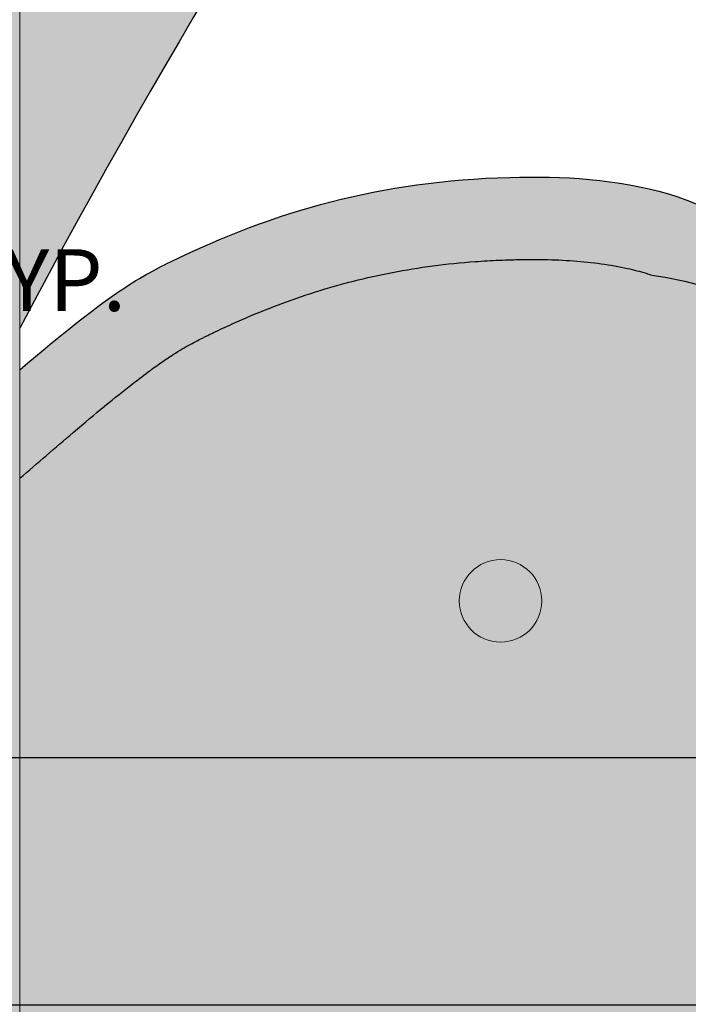
# Model space of a CAD drawing. Units: millimetres. Extents: x 11032 to 26788, y 3406 to 24505.
# Tile 72 of 78: x 22897 to 24519, y 12721 to 15110. Entities that reach past the tile are written whole.
import ezdxf

# ---------------------------------------------------------------- set-up
doc = ezdxf.new("R2010")
doc.units = ezdxf.units.MM
doc.header["$MEASUREMENT"] = 0
for name, color, linetype, lineweight in [('A-ANNO-DIMS', 2, 'Continuous', 18), ('A-GLAZ', 250, 'Continuous', 20), ('A-ROOF', 7, 'Continuous', 30), ('E-LITE', 7, 'Continuous', 18), ('E-LITE-PATT', 7, 'Continuous', 13)]:
    doc.layers.add(name, color=color, linetype=linetype, lineweight=lineweight)
for name, color, linetype, lineweight, true_color in [('A-GLAZ-FRAM-PATT', 250, 'Continuous', 13, 0x262627), ('A-ROOF-PATT', 9, 'Continuous', 13, 0xc7c8ca), ('A-WALL-CLAD-PATT', 9, 'Continuous', 13, 0xc7c8ca)]:
    doc.layers.add(name, color=color, linetype=linetype, lineweight=lineweight, true_color=true_color)
doc.styles.get("Standard").update_dxf_attribs({"font": 'arial.ttf'})
doc.dimstyles.get("Standard").update_dxf_attribs({"dimtxt": 150, "dimasz": 100, "dimexe": 10, "dimexo": 5, "dimgap": 5, "dimtad": 0, "dimtih": 1, "dimtoh": 1, "dimdec": 0, "dimzin": 0, "dimdsep": 46, "dimtxsty": 'Standard', "dimcen": 0.09, "dimadec": 0, "dimazin": 0, "dimtfac": 1, "dimtdec": 0, "dimtofl": 0, "dimtmove": 0, "dimatfit": 3, "dimfxl": 1, "dimtolj": 1, "dimtzin": 0, "dimarcsym": 0})

# ---------------------------------------------------------------- blocks, each defined once
blk = doc.blocks.new('RECESSED-LIGHT-200')
blk.add_circle((100, 100), 100)
blk = doc.blocks.new('*D20')
at = {"layer": 'A-ANNO-DIMS', "color": 0, "lineweight": -2, "transparency": 16777216}
for p, q in [((21468.9, 12413.4), (21368.9, 12413.4)), ((21568.9, 12403.4), (21568.9, 12423.4)), ((21668.9, 12403.4), (21668.9, 12423.4)), ((21768.9, 12413.4), (21868.9, 12413.4))]:
    blk.add_line(p, q, dxfattribs=at)
at = {"layer": 'A-ANNO-DIMS', "color": 0, "transparency": 16777216}
for points in [[(21468.9, 12430), (21468.9, 12396.7), (21568.9, 12413.4)], [(21768.9, 12430), (21768.9, 12396.7), (21668.9, 12413.4)]]:
    blk.add_solid(points, dxfattribs=at)
at = {"layer": 'Defpoints', "color": 0, "transparency": 16777216}
for p in [(21668.9, 12413.4), (21568.9, 12398.4), (21668.9, 12398.4)]:
    blk.add_point(p, dxfattribs=at)
at = {"layer": 'A-ANNO-DIMS', "color": 0, "transparency": 16777216, "insert": (23236.5, 12413.4), "char_height": 150, "attachment_point": 5}
blk.add_mtext('\\A1;RECESSED LIGHT 100 TYP.', dxfattribs=at)
blk = doc.blocks.new('*D22')
at = {"layer": 'A-ANNO-DIMS', "color": 0, "lineweight": -2, "transparency": 16777216}
for p, q in [((20094.7, 14478.3), (19994.7, 14478.3)), ((20194.7, 14460.8), (20194.7, 14488.3)), ((20344.7, 14460.8), (20344.7, 14488.3)), ((20444.7, 14478.3), (20544.7, 14478.3))]:
    blk.add_line(p, q, dxfattribs=at)
at = {"layer": 'A-ANNO-DIMS', "color": 0, "transparency": 16777216}
for points in [[(20094.7, 14495), (20094.7, 14461.7), (20194.7, 14478.3)], [(20444.7, 14495), (20444.7, 14461.7), (20344.7, 14478.3)]]:
    blk.add_solid(points, dxfattribs=at)
at = {"layer": 'Defpoints', "color": 0, "transparency": 16777216}
for p in [(20344.7, 14478.3), (20194.7, 14455.8), (20344.7, 14455.8)]:
    blk.add_point(p, dxfattribs=at)
at = {"layer": 'A-ANNO-DIMS', "color": 0, "transparency": 16777216, "insert": (21912.3, 14478.3), "char_height": 150, "attachment_point": 5}
blk.add_mtext('\\A1;RECESSED LIGHT 150 TYP.', dxfattribs=at)
blk = doc.blocks.new('*D36')
at = {"layer": 'A-ANNO-DIMS', "color": 0, "lineweight": -2, "transparency": 16777216}
for p, q in [((12301.3, 17115.9), (12301.3, 24416.9)), ((12401.3, 24406.9), (18569.2, 24406.9)), ((25297.4, 24406.9), (19129.5, 24406.9)), ((25397.4, 4466.4), (25397.4, 24416.9))]:
    blk.add_line(p, q, dxfattribs=at)
at = {"layer": 'A-ANNO-DIMS', "color": 0, "transparency": 16777216}
for points in [[(12401.3, 24423.5), (12401.3, 24390.2), (12301.3, 24406.9)], [(25297.4, 24423.5), (25297.4, 24390.2), (25397.4, 24406.9)]]:
    blk.add_solid(points, dxfattribs=at)
at = {"layer": 'Defpoints', "color": 0, "transparency": 16777216}
for p in [(25397.4, 24406.9), (12301.3, 17110.9), (25397.4, 4461.4)]:
    blk.add_point(p, dxfattribs=at)
at = {"layer": 'A-ANNO-DIMS', "color": 0, "transparency": 16777216, "insert": (18849.3, 24406.9), "char_height": 150, "attachment_point": 5}
blk.add_mtext('\\A1;13096', dxfattribs=at)
blk = doc.blocks.new('*D42')
at = {"layer": 'A-ANNO-DIMS', "color": 0, "lineweight": -2, "transparency": 16777216}
for p, q in [((22752.4, 13320.1), (26363.9, 13320.1)), ((26353.9, 13220.1), (26353.9, 13101.7)), ((26353.9, 12820.1), (26353.9, 12938.5)), ((22752.4, 12720.1), (26363.9, 12720.1))]:
    blk.add_line(p, q, dxfattribs=at)
at = {"layer": 'A-ANNO-DIMS', "color": 0, "transparency": 16777216}
for points in [[(26337.2, 13220.1), (26370.6, 13220.1), (26353.9, 13320.1)], [(26337.2, 12820.1), (26370.6, 12820.1), (26353.9, 12720.1)]]:
    blk.add_solid(points, dxfattribs=at)
at = {"layer": 'Defpoints', "color": 0, "transparency": 16777216}
for p in [(22747.4, 13320.1), (26353.9, 13320.1), (22747.4, 12720.1)]:
    blk.add_point(p, dxfattribs=at)
at = {"layer": 'A-ANNO-DIMS', "color": 0, "transparency": 16777216, "insert": (26353.9, 13020.1), "char_height": 150, "attachment_point": 5}
blk.add_mtext('\\A1;600', dxfattribs=at)
blk = doc.blocks.new('*D43')
at = {"layer": 'A-ANNO-DIMS', "color": 0, "lineweight": -2, "transparency": 16777216}
for p, q in [((22752.4, 15170.1), (26363.9, 15170.1)), ((26353.9, 15070.1), (26353.9, 14326.7)), ((26353.9, 13420.1), (26353.9, 14163.5)), ((22752.4, 13320.1), (26363.9, 13320.1))]:
    blk.add_line(p, q, dxfattribs=at)
at = {"layer": 'A-ANNO-DIMS', "color": 0, "transparency": 16777216}
for points in [[(26337.2, 15070.1), (26370.6, 15070.1), (26353.9, 15170.1)], [(26337.2, 13420.1), (26370.6, 13420.1), (26353.9, 13320.1)]]:
    blk.add_solid(points, dxfattribs=at)
at = {"layer": 'Defpoints', "color": 0, "transparency": 16777216}
for p in [(22747.4, 15170.1), (26353.9, 15170.1), (22747.4, 13320.1)]:
    blk.add_point(p, dxfattribs=at)
at = {"layer": 'A-ANNO-DIMS', "color": 0, "transparency": 16777216, "insert": (26353.9, 14245.1), "char_height": 150, "attachment_point": 5}
blk.add_mtext('\\A1;1850', dxfattribs=at)

msp = doc.modelspace()

# ---------------------------------------------------------------- hatches: boundary and pattern name
at = {"layer": 'A-GLAZ-FRAM-PATT'}
h = msp.add_hatch(color=256, dxfattribs=at)
h.paths.add_polyline_path([(22747.404, 16218.44), (22395.025, 16218.44), (18518.2, 16200.148), (18519.143, 16000.151), (22747.404, 16020.1)])
edge = h.paths.add_edge_path()
edge.add_line((22897.404, 16218.44), (22747.404, 16218.44))
edge.add_line((22747.404, 16218.44), (22747.404, 16020.1))
edge.add_line((22747.404, 16020.1), (22747.404, 9631.346))
edge.add_spline(control_points=[(22747.404, 9631.346), (22803.273, 9520.228), (22853.467, 9405.87), (22897.404, 9289.211)], knot_values=[2645.78092422, 2645.78092422, 2645.78092422, 2645.78092422, 3013.05623672, 3013.05623672, 3013.05623672, 3013.05623672], degree=3, periodic=0)
edge.add_line((22897.404, 9289.211), (22897.404, 16218.44))
h.paths.add_polyline_path([(22097.404, 16017.033), (21997.404, 16016.562), (21997.404, 13316.532), (22097.404, 13317.003)])
edge = h.paths.add_edge_path()
edge.add_line((19797.404, 16006.182), (19697.404, 16005.71))
edge.add_line((19697.404, 16005.71), (19697.404, 15155.703))
edge.add_line((19697.404, 15155.703), (19697.404, 12747.012))
edge.add_spline(control_points=[(19697.404, 12747.012), (19708.389, 12750.081), (19719.253, 12753.406), (19732.457, 12757.789), (19734.918, 12758.62), (19737.372, 12759.464)], knot_values=[1372.60477099, 1372.60477099, 1372.60477099, 1372.60477099, 1399.44343377, 1399.44343377, 1405.61279972, 1405.61279972, 1405.61279972, 1405.61279972], degree=3, periodic=0)
edge.add_spline(control_points=[(19737.372, 12759.464), (19750.245, 12763.891), (19762.932, 12768.657), (19778.9, 12775.14), (19782.354, 12776.572), (19785.794, 12778.028)], knot_values=[1405.61279972, 1405.61279972, 1405.61279972, 1405.61279972, 1437.96891336, 1437.96891336, 1446.94640473, 1446.94640473, 1446.94640473, 1446.94640473], degree=3, periodic=0)
edge.add_spline(control_points=[(19785.794, 12778.028), (19789.682, 12779.673), (19793.552, 12781.348), (19797.404, 12783.051)], knot_values=[1446.94640473, 1446.94640473, 1446.94640473, 1446.94640473, 1457.09545574, 1457.09545574, 1457.09545574, 1457.09545574], degree=3, periodic=0)
edge.add_line((19797.404, 12783.051), (19797.404, 15306.174))
edge.add_line((19797.404, 15306.174), (19797.404, 16006.182))
at = {"layer": 'A-ROOF-PATT'}
h = msp.add_hatch(color=256, dxfattribs=at)
h.set_gradient(color1=(254, 234, 185), color2=(254, 204, 102), name='HEMISPHERICAL')
edge = h.paths.add_edge_path()
edge.add_line((22395.025, 16218.44), (22897.404, 16218.44))
edge.add_line((22897.404, 16218.44), (22897.404, 14361.22))
edge.add_spline(control_points=[(22897.404, 14361.22), (23633.498, 15762.375), (24369.592, 16638.387), (24279.347, 17098.191)], knot_values=[13837.11981978, 13837.11981978, 13837.11981978, 13837.11981978, 16370.50452639, 16370.50452639, 16370.50452639, 16370.50452639], degree=3, periodic=0)
edge.add_spline(control_points=[(24279.347, 17098.191), (24257.37, 17136.735), (24193.084, 17226.949), (23988.629, 17323.661), (23687.5, 17400.339), (23443.416, 17391.278), (23304.873, 17403.391)], knot_values=[0, 0, 0, 0, 132.15616417, 336.8260172, 651.2646938, 1064.01641738, 1064.01641738, 1064.01641738, 1064.01641738], degree=3, periodic=0)
edge.add_spline(control_points=[(23304.873, 17403.391), (23244.326, 17403.734), (23179.968, 17412.17), (23070.675, 17406.134), (23026.355, 17412.719), (22981.194, 17409.426)], knot_values=[11756.28081343, 11756.28081343, 11756.28081343, 11756.28081343, 11943.0031739, 11943.0031739, 12065.87545546, 12065.87545546, 12065.87545546, 12065.87545546], degree=3, periodic=0)
edge.add_spline(control_points=[(22981.194, 17409.426), (22912.577, 17410.967), (22705.353, 17409.356), (22364.272, 17406.622), (21915.866, 17351.508), (21440.234, 17310.172), (20910.567, 17150.246), (20408.011, 17091.181), (20122.484, 17046.068), (19965.955, 17031.58)], knot_values=[0, 0, 0, 0, 192.80748108, 571.75839709, 1088.96543094, 1535.73720072, 2007.04970373, 2677.45974628, 3092.27759325, 3092.27759325, 3092.27759325, 3092.27759325], degree=3, periodic=0)
edge.add_spline(control_points=[(19965.955, 17031.58), (19761.843, 17020.464), (19288.07, 16988.339), (18809.773, 17038.521), (18514.126, 17063.566)], knot_values=[0, 0, 0, 0, 511.7030916, 1383.18424693, 1383.18424693, 1383.18424693, 1383.18424693], degree=3, periodic=0)
edge.add_line((18514.126, 17063.566), (18518.2, 16200.148))
edge.add_line((18518.2, 16200.148), (22395.025, 16218.44))
h.paths.add_polyline_path([(20159.481, 16629.671, -1), (20359.481, 16629.671, -1)], flags=16)
h.paths.add_polyline_path([(22641.869, 16640.848, -1), (22441.869, 16640.848, -1)], flags=16)
h.paths.add_polyline_path([(23436.23, 16026.079, -1), (23236.23, 16026.079, -1)], flags=16)
h = msp.add_hatch(color=256, dxfattribs=at)
h.set_gradient(color1=(254, 234, 185), color2=(254, 204, 102), name='HEMISPHERICAL')
edge = h.paths.add_edge_path()
edge.add_spline(control_points=[(22897.404, 11669.966), (22905.925, 11665.421), (23315.936, 11448.075), (24040.798, 11159.928), (24591.756, 12047.169), (24823.737, 12810.982), (24947.403, 13888.961), (24865.187, 14241.353)], knot_values=[3287.74811127, 3287.74811127, 3287.74811127, 3287.74811127, 3313.95061448, 4543.69878516, 5160.49832431, 6201.61230094, 7164.26935092, 7164.26935092, 7164.26935092, 7164.26935092], degree=3, periodic=0)
edge.add_spline(control_points=[(24865.187, 14241.353), (24864.423, 14242.575), (24766.311, 14398.016), (24602.876, 14465.087), (24430.499, 14490.269)], knot_values=[2462.20964139, 2462.20964139, 2462.20964139, 2462.20964139, 2466.8266732, 3052.28296943, 3052.28296943, 3052.28296943, 3052.28296943], degree=3, periodic=0)
edge.add_spline(control_points=[(24430.499, 14490.269), (24425.883, 14491.82), (24421.191, 14493.323), (24402.038, 14499.174), (24386.985, 14503.129), (24351.089, 14511.181), (24329.855, 14514.969), (24285.944, 14521.074), (24263.27, 14523.392), (24216.998, 14526.696), (24193.401, 14527.682), (24156.534, 14528.34), (24143.408, 14528.404), (24117.112, 14528.234), (24103.938, 14528.001), (24070.613, 14527.088), (24050.758, 14526.245), (24021.415, 14524.553), (24011.706, 14523.918), (23966.994, 14520.648), (23932.846, 14517.154), (23866.075, 14508.38), (23833.453, 14503.099), (23769.399, 14490.798), (23737.967, 14483.778), (23675.954, 14468.02), (23645.373, 14459.282), (23584.735, 14440.092), (23554.677, 14429.638), (23494.779, 14407.002), (23464.938, 14394.819), (23420.13, 14375.236), (23405.186, 14368.49), (23382.735, 14358.043), (23375.245, 14354.506), (23363.999, 14349.118), (23360.248, 14347.308), (23354.645, 14344.586), (23352.794, 14343.684), (23350.017, 14342.326), (23349.099, 14341.876), (23346.705, 14340.7), (23345.24, 14339.978), (23338.743, 14336.765), (23333.903, 14334.336), (23322.952, 14328.714), (23316.906, 14325.517), (23304.544, 14318.72), (23298.224, 14315.118), (23284.755, 14307.106), (23277.606, 14302.694), (23262.032, 14292.682), (23253.61, 14287.081), (23235.154, 14274.351), (23225.122, 14267.224), (23200.911, 14249.486), (23186.304, 14238.46), (23150.266, 14210.435), (23128.041, 14192.649), (23080.227, 14153.32), (23055.083, 14132.223), (23027.357, 14108.523)], knot_values=[765.02120011, 765.02120011, 765.02120011, 765.02120011, 788.26421035, 788.26421035, 858.47024111, 858.47024111, 949.55129088, 949.55129088, 1040.63234064, 1040.63234064, 1131.71339041, 1131.71339041, 1181.69353236, 1181.69353236, 1231.67367431, 1231.67367431, 1308.31901537, 1308.31901537, 1346.64168591, 1346.64168591, 1486.09404767, 1486.09404767, 1625.54640943, 1625.54640943, 1764.99877119, 1764.99877119, 1904.45113295, 1904.45113295, 2043.90349471, 2043.90349471, 2183.35585648, 2183.35585648, 2253.08203736, 2253.08203736, 2287.9451278, 2287.9451278, 2305.37667302, 2305.37667302, 2313.97014819, 2313.97014819, 2318.26688578, 2318.26688578, 2325.26983634, 2325.26983634, 2349.68341829, 2349.68341829, 2381.60377634, 2381.60377634, 2413.52413439, 2413.52413439, 2445.44449243, 2445.44449243, 2477.36485048, 2477.36485048, 2509.28520853, 2509.28520853, 2547.80727814, 2547.80727814, 2595.07704725, 2595.07704725, 2638.35089074, 2638.35089074, 2638.35089074, 2638.35089074], degree=3, periodic=0)
edge.add_spline(control_points=[(23027.357, 14108.523), (23027.349, 14108.516), (23027.342, 14108.51), (23027.334, 14108.504), (22984.024, 14071.482), (22940.714, 14034.46), (22897.404, 13997.439)], knot_values=[697.41436256, 697.41436256, 697.41436256, 697.41436256, 697.4261083, 697.4261083, 697.4261083, 765.02120011, 765.02120011, 765.02120011, 765.02120011], degree=3, periodic=0)
edge.add_line((22897.404, 13997.439), (22897.404, 11669.966))
h.paths.add_polyline_path([(23729.349, 12537.488, -1), (23529.349, 12537.488, -1)], flags=16)
h.paths.add_polyline_path([(23963.611, 13699.89, -1), (24163.611, 13699.89, -1)], flags=16)
at = {"layer": 'A-WALL-CLAD-PATT'}
h = msp.add_hatch(color=256, dxfattribs=at)
edge = h.paths.add_edge_path()
edge.add_spline(control_points=[(24865.187, 14241.353), (24844.683, 14329.238), (24708.481, 14689.762), (23980.011, 14777.842), (23439.65, 14624.598), (23111.535, 14443.589), (22897.404, 14260.55)], knot_values=[765.02120011, 765.02120011, 765.02120011, 765.02120011, 1005.10337375, 1880.54593672, 2963.32805357, 3287.74811127, 3287.74811127, 3287.74811127, 3287.74811127], degree=3, periodic=0)
edge.add_line((22897.404, 14260.55), (22897.404, 13997.439))
edge.add_spline(control_points=[(22897.404, 13997.439), (22940.714, 14034.46), (22984.024, 14071.482), (23027.334, 14108.504), (23027.342, 14108.51), (23027.349, 14108.516), (23027.357, 14108.523)], knot_values=[697.41436256, 697.41436256, 697.41436256, 697.41436256, 765.00945437, 765.00945437, 765.00945437, 765.02120011, 765.02120011, 765.02120011, 765.02120011], degree=3, periodic=0)
edge.add_spline(control_points=[(23027.357, 14108.523), (23055.083, 14132.223), (23080.227, 14153.32), (23128.041, 14192.649), (23150.266, 14210.435), (23186.304, 14238.46), (23200.911, 14249.486), (23225.122, 14267.224), (23235.154, 14274.351), (23253.61, 14287.081), (23262.032, 14292.682), (23277.606, 14302.694), (23284.755, 14307.106), (23298.224, 14315.118), (23304.544, 14318.72), (23316.906, 14325.517), (23322.952, 14328.714), (23333.903, 14334.336), (23338.743, 14336.765), (23345.24, 14339.978), (23346.705, 14340.7), (23349.099, 14341.876), (23350.017, 14342.326), (23352.794, 14343.684), (23354.645, 14344.586), (23360.248, 14347.308), (23363.999, 14349.118), (23375.245, 14354.506), (23382.735, 14358.043), (23405.186, 14368.49), (23420.13, 14375.236), (23464.938, 14394.819), (23494.779, 14407.002), (23554.677, 14429.638), (23584.735, 14440.092), (23645.373, 14459.282), (23675.954, 14468.02), (23737.967, 14483.778), (23769.399, 14490.798), (23833.453, 14503.099), (23866.075, 14508.38), (23932.846, 14517.154), (23966.994, 14520.648), (24011.706, 14523.918), (24021.415, 14524.553), (24050.758, 14526.245), (24070.613, 14527.088), (24103.938, 14528.001), (24117.112, 14528.234), (24143.408, 14528.404), (24156.534, 14528.34), (24193.401, 14527.682), (24216.998, 14526.696), (24263.27, 14523.392), (24285.944, 14521.074), (24329.855, 14514.969), (24351.089, 14511.181), (24386.985, 14503.129), (24402.038, 14499.174), (24421.191, 14493.323), (24425.883, 14491.82), (24430.499, 14490.269)], knot_values=[765.02120011, 765.02120011, 765.02120011, 765.02120011, 808.29504361, 808.29504361, 855.56481272, 855.56481272, 894.08688233, 894.08688233, 926.00724037, 926.00724037, 957.92759842, 957.92759842, 989.84795647, 989.84795647, 1021.76831451, 1021.76831451, 1053.68867256, 1053.68867256, 1078.10225451, 1078.10225451, 1085.10520508, 1085.10520508, 1089.40194266, 1089.40194266, 1097.99541784, 1097.99541784, 1115.42696306, 1115.42696306, 1150.2900535, 1150.2900535, 1220.01623438, 1220.01623438, 1359.46859614, 1359.46859614, 1498.9209579, 1498.9209579, 1638.37331966, 1638.37331966, 1777.82568142, 1777.82568142, 1917.27804319, 1917.27804319, 2056.73040495, 2056.73040495, 2095.05307548, 2095.05307548, 2171.69841654, 2171.69841654, 2221.67855849, 2221.67855849, 2271.65870045, 2271.65870045, 2362.73975021, 2362.73975021, 2453.82079998, 2453.82079998, 2544.90184974, 2544.90184974, 2615.10788051, 2615.10788051, 2638.35089074, 2638.35089074, 2638.35089074, 2638.35089074], degree=3, periodic=0)
edge.add_spline(control_points=[(24430.499, 14490.269), (24602.876, 14465.087), (24766.311, 14398.016), (24864.423, 14242.575), (24865.187, 14241.353)], knot_values=[2462.20964139, 2462.20964139, 2462.20964139, 2462.20964139, 3047.66593763, 3052.28296943, 3052.28296943, 3052.28296943, 3052.28296943], degree=3, periodic=0)
h.paths.add_polyline_path([(25397.404, 11120.753), (22897.404, 11120.753), (22897.404, 10520.753), (25197.404, 10520.753), (25197.404, 9359.601), (25397.404, 9359.601)])
at = {"layer": 'E-LITE-PATT'}
h = msp.add_hatch(color=256, dxfattribs=at)
h.paths.add_polyline_path([(23729.349, 12537.488, 1), (23529.349, 12537.488, 1)])
h.paths.add_polyline_path([(24163.611, 13699.89, 1), (23963.611, 13699.89, 1)])
h.paths.add_polyline_path([(18790.086, 14298.34, 1), (18890.086, 14298.34, 1)])
h.paths.add_polyline_path([(19537.524, 14550.125, 1), (19437.524, 14550.125, 1)])
h.paths.add_polyline_path([(20194.664, 14380.821, 1), (20344.664, 14380.821, 1)])
h.paths.add_polyline_path([(20018.772, 14780.204, 1), (19868.772, 14780.204, 1)])
h.paths.add_polyline_path([(20594.425, 14224.541, 1), (20744.425, 14224.541, 1)])
h.paths.add_polyline_path([(21232.101, 14202.835, 1), (21332.101, 14202.835, 1)])
h.paths.add_polyline_path([(20854.127, 14602.218, 1), (20754.127, 14602.218, 1)])
h.paths.add_polyline_path([(21492.875, 14667.335, 1), (21392.875, 14667.335, 1)])
h.paths.add_polyline_path([(21005.138, 14988.578, 1), (20855.138, 14988.578, 1)])
h = msp.add_hatch(color=256, dxfattribs=at)
h.paths.add_polyline_path([(21120.849, 11395.371, 1), (21220.849, 11395.371, 1)])
h.paths.add_polyline_path([(21215.053, 11595.746, 1), (21315.053, 11595.746, 1)])
h.paths.add_polyline_path([(21407.506, 11792.395, 1), (21307.506, 11792.395, 1)])
h.paths.add_polyline_path([(21507.11, 12004.255, 1), (21407.11, 12004.255, 1)])
h.paths.add_polyline_path([(21501.367, 12204.741, 1), (21601.367, 12204.741, 1)])
h.paths.add_polyline_path([(21668.897, 12348.379, 1), (21568.897, 12348.379, 1)])
h.paths.add_polyline_path([(23729.349, 12537.488, 1), (23529.349, 12537.488, 1)])
h.paths.add_polyline_path([(23963.611, 13699.89, 1), (24163.611, 13699.89, 1)])
h.paths.add_polyline_path([(21492.875, 14667.335, 1), (21392.875, 14667.335, 1)])
h.paths.add_polyline_path([(21332.101, 14202.835, 1), (21232.101, 14202.835, 1)])
h.paths.add_polyline_path([(20744.425, 14224.541, 1), (20594.425, 14224.541, 1)])
h.paths.add_polyline_path([(20854.127, 14602.218, 1), (20754.127, 14602.218, 1)])
h.paths.add_polyline_path([(20947.253, 15061.599), (20912.335, 15061.434, 0.34563694), (20855.138, 14988.578, 1), (21005.138, 14988.578, 0.34827999)])
h = msp.add_hatch(color=256, dxfattribs=at)
h.paths.add_polyline_path([(23529.349, 12537.488, 1), (23729.349, 12537.488, 1)])
h.paths.add_polyline_path([(24163.611, 13699.89, 1), (23963.611, 13699.89, 1)])

# ---------------------------------------------------------------- linework, layer by layer
at = {"layer": 'A-GLAZ'}
msp.add_line((22897.404, 16218.44), (22897.404, 9289.211), dxfattribs=at)
at = {"layer": 'A-ROOF'}
for points, knots in [([(19305.291, 17259.568), (19382.851, 17264.718), (19460.41, 17269.868), (19537.97, 17275.018), (19654.15, 17282.732), (19770.33, 17290.447), (19886.51, 17298.161), (19886.51, 17298.161), (19886.51, 17298.161), (19886.51, 17298.161), (20092.886, 17311.864), (21679.83, 17482.933), (25498.5, 17958.124), (23655.645, 15804.534), (22897.404, 14361.22)], [8878.9087223, 8878.9087223, 8878.9087223, 8878.9087223, 9101.65833771, 9101.65833771, 9101.65833771, 9435.32303857, 9435.32303857, 9435.32303857, 9435.32329041, 9435.32329041, 9435.32329041, 10028.02667108, 13760.8945204, 16370.50452639, 16370.50452639, 16370.50452639, 16370.50452639]), ([(22897.404, 14260.55), (23111.535, 14443.589), (23439.65, 14624.598), (23980.011, 14777.842), (25027.484, 14651.191), (24844.989, 12880.959), (24591.756, 12047.169), (24040.798, 11159.928), (23315.936, 11448.075), (22905.925, 11665.421), (22897.404, 11669.966)], [765.02120011, 765.02120011, 765.02120011, 765.02120011, 1089.44125781, 2172.22337467, 3047.66593763, 4250.40516126, 5291.51913789, 5908.31867703, 7138.06684772, 7164.26935092, 7164.26935092, 7164.26935092, 7164.26935092]), ([(22897.404, 13997.439), (22940.714, 14034.46), (22984.024, 14071.482), (23027.334, 14108.504), (23027.342, 14108.51), (23027.349, 14108.516), (23027.357, 14108.523), (23055.083, 14132.223), (23080.227, 14153.32), (23128.041, 14192.649), (23150.266, 14210.435), (23186.304, 14238.46), (23200.911, 14249.486), (23225.122, 14267.224), (23235.154, 14274.351), (23253.61, 14287.081), (23262.032, 14292.682), (23277.606, 14302.694), (23284.755, 14307.106), (23298.224, 14315.118), (23304.544, 14318.72), (23316.906, 14325.517), (23322.952, 14328.714), (23333.903, 14334.336), (23338.743, 14336.765), (23345.24, 14339.978), (23346.705, 14340.7), (23349.099, 14341.876), (23350.017, 14342.326), (23352.794, 14343.684), (23354.645, 14344.586), (23360.248, 14347.308), (23363.999, 14349.118), (23375.245, 14354.506), (23382.735, 14358.043), (23405.186, 14368.49), (23420.13, 14375.236), (23464.938, 14394.819), (23494.779, 14407.002), (23554.677, 14429.638), (23584.735, 14440.092), (23645.373, 14459.282), (23675.954, 14468.02), (23737.967, 14483.778), (23769.399, 14490.798), (23833.453, 14503.099), (23866.075, 14508.38), (23932.846, 14517.154), (23966.994, 14520.648), (24011.706, 14523.918), (24021.415, 14524.553), (24050.758, 14526.245), (24070.613, 14527.088), (24103.938, 14528.001), (24117.112, 14528.234), (24143.408, 14528.404), (24156.534, 14528.34), (24193.401, 14527.682), (24216.998, 14526.696), (24263.27, 14523.392), (24285.944, 14521.074), (24329.855, 14514.969), (24351.089, 14511.181), (24386.985, 14503.129), (24402.038, 14499.174), (24421.191, 14493.323), (24425.883, 14491.82), (24430.499, 14490.269)], [697.41436256, 697.41436256, 697.41436256, 697.41436256, 765.00945437, 765.00945437, 765.00945437, 765.02120011, 765.02120011, 765.02120011, 808.29504361, 808.29504361, 855.56481272, 855.56481272, 894.08688233, 894.08688233, 926.00724037, 926.00724037, 957.92759842, 957.92759842, 989.84795647, 989.84795647, 1021.76831451, 1021.76831451, 1053.68867256, 1053.68867256, 1078.10225451, 1078.10225451, 1085.10520508, 1085.10520508, 1089.40194266, 1089.40194266, 1097.99541784, 1097.99541784, 1115.42696306, 1115.42696306, 1150.2900535, 1150.2900535, 1220.01623438, 1220.01623438, 1359.46859614, 1359.46859614, 1498.9209579, 1498.9209579, 1638.37331966, 1638.37331966, 1777.82568142, 1777.82568142, 1917.27804319, 1917.27804319, 2056.73040495, 2056.73040495, 2095.05307548, 2095.05307548, 2171.69841654, 2171.69841654, 2221.67855849, 2221.67855849, 2271.65870045, 2271.65870045, 2362.73975021, 2362.73975021, 2453.82079998, 2453.82079998, 2544.90184974, 2544.90184974, 2615.10788051, 2615.10788051, 2638.35089074, 2638.35089074, 2638.35089074, 2638.35089074]), ([(24430.499, 14490.269), (24602.876, 14465.087), (24766.311, 14398.016), (24864.423, 14242.575), (24865.187, 14241.353)], [2462.20964139, 2462.20964139, 2462.20964139, 2462.20964139, 3047.66593763, 3052.28296943, 3052.28296943, 3052.28296943, 3052.28296943])]:
    msp.add_open_spline(points, degree=3, knots=knots, dxfattribs=at)

# ---------------------------------------------------------------- block references
at = {"layer": 'E-LITE'}
msp.add_blockref('RECESSED-LIGHT-200', (23963.611, 13599.89), dxfattribs=at)

# ---------------------------------------------------------------- dimensions: what is measured, and where the dimension line sits
at = {"layer": 'A-ANNO-DIMS'}
dim = msp.add_linear_dim(base=(25397.404, 24406.858), p1=(12301.265, 17110.885), p2=(25397.404, 4461.399), dimstyle='Standard', override={"dimdec": 0, "dimlfac": 1, "dimrnd": 0, "dimzin": 0, "dimdsep": 46, "dimlunit": 2}, dxfattribs=at)
dim.commit()
dim.dimension.update_dxf_attribs({"geometry": '*D36', "text_midpoint": (18849.334, 24406.858)})
for base, p1, p2, picture, middle in [((26353.904, 15170.094), (22747.404, 13320.07), (22747.404, 15170.094), '*D43', (26353.904, 14245.082)), ((26353.904, 13320.07), (22747.404, 12720.064), (22747.404, 13320.07), '*D42', (26353.904, 13020.067))]:
    dim = msp.add_linear_dim(base=base, p1=p1, p2=p2, angle=90, dimstyle='Standard', override={"dimdec": 0, "dimlfac": 1, "dimrnd": 0, "dimzin": 0, "dimdsep": 46, "dimlunit": 2}, dxfattribs=at)
    dim.commit()
    dim.dimension.update_dxf_attribs({"geometry": picture, "text_midpoint": middle})
for base, p1, p2, picture, middle in [((20344.664, 14478.321), (20194.664, 14455.821), (20344.664, 14455.821), '*D22', (21912.301, 14478.321)), ((21668.897, 12413.379), (21568.897, 12398.379), (21668.897, 12398.379), '*D20', (23236.534, 12413.379))]:
    dim = msp.add_linear_dim(base=base, p1=p1, p2=p2, text='RECESSED LIGHT <> TYP.', dimstyle='Standard', override={"dimdec": 0, "dimlfac": 1, "dimrnd": 0, "dimzin": 0, "dimdsep": 46, "dimlunit": 2}, dxfattribs=at)
    dim.commit()
    dim.dimension.update_dxf_attribs({"geometry": picture, "text_midpoint": middle})

doc.saveas('drawing.dxf')
